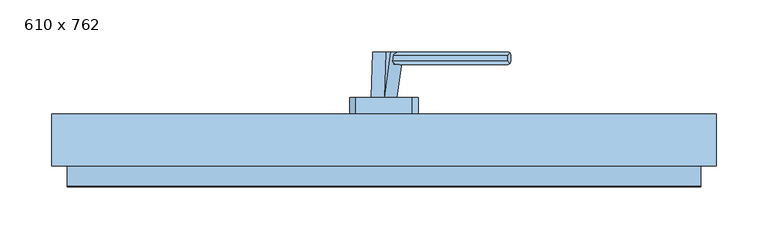
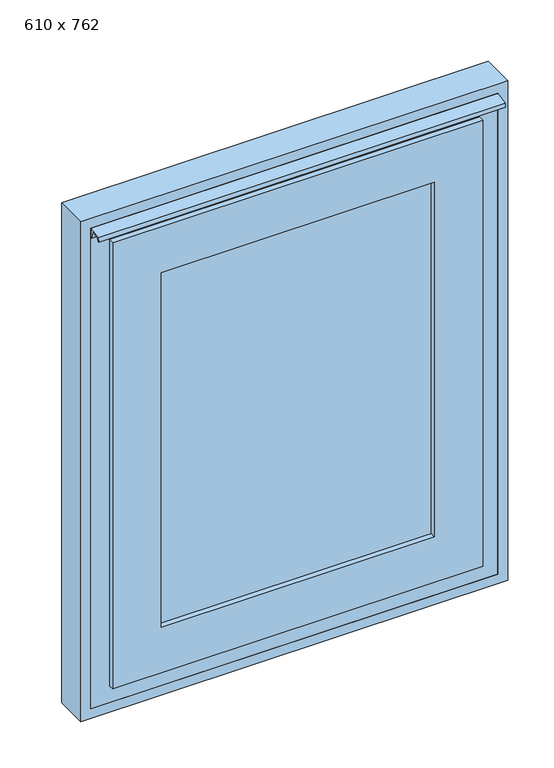
"""IFC4 building model written with IfcOpenShell, lengths in millimetres: window geometry, 610 x 762."""

from ifc_helpers import new_model, si_unit, point, frame, frame_2d, origin, place, context, project, spatial, polyline, circle_curve, ellipse_curve, trimmed, segment, composite_curve, outline, extrude, faceted_brep, source, transform, mapped, element, save
from ifc_brep_helpers import plane_surface, cylinder_surface, extruded_surface, advanced_brep


def window_610_x_762_5077743b(model_context):
    return source(origin(), model_context, "Body", "SolidModel", [
        advanced_brep(
        [(6.2046905, 15.7, 888.0038591), (6.2046905, 15.7, 863.0038591), (1.7209614, 15.7, 863.0038591), (1.7209614, 15.7, 888.0038591), (0.0, -28.3, 888.0038591), (0.0, -28.3, 863.0038591)],
        [
            (0, 1, circle_curve(frame((6.2046905, 15.7, 875.5038591), z_axis=(0.0, 1.0, 0.0), x_axis=(1.0, 0.0, 0.0)), 12.5)),
            (1, 2),
            (2, 3, circle_curve(frame((1.7209614, 15.7, 875.5038591), z_axis=(0.0, 1.0, 0.0), x_axis=(1.0, 0.0, 0.0)), 12.5)),
            (3, 0),
            (4, 5, circle_curve(frame((0.0, -28.3, 875.5038591), z_axis=(0.0, -1.0, 0.0), x_axis=(1.0, 0.0, 0.0)), 12.5)),
            (5, 4, circle_curve(frame((0.0, -28.3, 875.5038591), z_axis=(0.0, -1.0, 0.0), x_axis=(1.0, 0.0, 0.0)), 12.5)),
            (4, 3),
            (2, 5),
            (4, 0),
            (1, 5),
        ],
        [
            plane_surface(frame((3.9628259, 15.7, 875.5038591), z_axis=(0.0, 1.0, 0.0), x_axis=(-1.0, 0.0, 0.0))),
            plane_surface(frame((0.0, -28.3, 875.5038591), z_axis=(0.0, -1.0, 0.0), x_axis=(-1.0, 0.0, 0.0))),
            extruded_surface(trimmed(circle_curve(frame((1.7209614, 15.7, 875.5038591), z_axis=(0.0, -1.0, 0.0), x_axis=(1.0, 0.0, 0.0)), 12.5), [point((1.7209614, 15.7, 888.0038591))], [point((1.7209614, 15.7, 863.0038591))], True, "CARTESIAN"), (-1.7209614, -44.0, 0.0), 44.03364291244014),
            plane_surface(frame((0.0, -28.3, 888.0038591), z_axis=(0.0, 0.0, 1.0), x_axis=(-1.0, 0.0, 0.0))),
            plane_surface(frame((0.0, -28.3, 863.0038591), z_axis=(0.0, 0.0, -1.0), x_axis=(1.0, 0.0, 0.0))),
            extruded_surface(trimmed(circle_curve(frame((6.2046905, 15.7, 875.5038591), z_axis=(0.0, -1.0, 0.0), x_axis=(1.0, 0.0, 0.0)), 12.5), [point((6.2046905, 15.7, 863.0038591))], [point((6.2046905, 15.7, 888.0038591))], True, "CARTESIAN"), (-6.2046905, -44.0, 0.0), 44.43532585905937),
        ],
        [
            (0, [[1, 2, 3, 4]]),
            (1, [[5, 6]]),
            (2, [[7, -3, 8, -5]]),
            (3, [[-7, 9, -4]]),
            (4, [[10, -8, -2]]),
            (5, [[-10, -1, -9, -6]]),
        ],
    ),
        advanced_brep(
        [(122.0, 12.7, 866.0038591), (122.0, 12.7, 885.0038591), (122.0, 6.7, 885.0038591), (122.0, 6.7, 866.0038591), (4.7741708, 15.7, 866.0038591), (113.6581962, 15.7, 866.0038591), (119.0, 15.7, 866.0038591), (121.1213203, 14.8213203, 863.8825388), (119.0, 12.7, 863.0038591), (110.9250215, 12.7, 863.0038591), (4.7741708, 12.7, 863.0038591), (4.7741708, 6.7, 863.0038591), (110.9250215, 6.7, 863.0038591), (119.0, 6.7, 863.0038591), (121.1213203, 4.5786797, 863.8825388), (119.0, 3.7, 866.0038591), (113.6581962, 3.7, 866.0038591), (4.7741708, 3.7, 866.0038591), (119.0, 3.7, 885.0038591), (113.6581962, 3.7, 885.0038591), (4.7741708, 3.7, 885.0038591), (121.1213203, 4.5786797, 887.1251795), (119.0, 6.7, 888.0038591), (110.9250215, 6.7, 888.0038591), (4.7741708, 6.7, 888.0038591), (4.7741708, 12.7, 888.0038591), (110.9250215, 12.7, 888.0038591), (119.0, 12.7, 888.0038591), (121.1213203, 14.8213203, 887.1251795), (119.0, 15.7, 885.0038591), (113.6581962, 15.7, 885.0038591), (4.7741708, 15.7, 885.0038591)],
        [
            (0, 1),
            (1, 2),
            (2, 3),
            (3, 0),
            (4, 5),
            (5, 6),
            (6, 7, ellipse_curve(frame((119.0, 12.7, 866.0038591), z_axis=(-0.70710678118655, 0.0, -0.7071067811865449), x_axis=(0.7071067811865451, 0.0, -0.7071067811865498)), 4.2426407, 3.0)),
            (7, 8, ellipse_curve(frame((119.0, 12.7, 866.0038591), z_axis=(-0.7071067811865427, 0.7071067811865525, 0.0), x_axis=(0.7071067811865522, 0.7071067811865428, 0.0)), 4.2426407, 3.0)),
            (8, 9),
            (9, 10),
            (10, 4, circle_curve(frame((4.7741708, 12.7, 866.0038591), z_axis=(1.0, 0.0, 0.0), x_axis=(0.0, 0.0, 1.0)), 3.0)),
            (11, 12),
            (12, 13),
            (13, 14, ellipse_curve(frame((119.0, 6.7, 866.0038591), z_axis=(-0.7071067811865523, -0.7071067811865426, 0.0), x_axis=(0.7071067811865428, -0.7071067811865522, 0.0)), 4.2426407, 3.0)),
            (14, 15, ellipse_curve(frame((119.0, 6.7, 866.0038591), z_axis=(-0.70710678118655, 0.0, -0.7071067811865449), x_axis=(0.7071067811865451, 0.0, -0.7071067811865498)), 4.2426407, 3.0)),
            (15, 16),
            (16, 17),
            (17, 11, circle_curve(frame((4.7741708, 6.7, 866.0038591), z_axis=(1.0, 0.0, 0.0), x_axis=(0.0, 0.0, 1.0)), 3.0)),
            (15, 18),
            (18, 19),
            (19, 20),
            (20, 17),
            (18, 21, ellipse_curve(frame((119.0, 6.7, 885.0038591), z_axis=(-0.7071067811865449, 0.0, 0.70710678118655), x_axis=(0.7071067811865501, 0.0, 0.7071067811865448)), 4.2426407, 3.0)),
            (21, 22, ellipse_curve(frame((119.0, 6.7, 885.0038591), z_axis=(-0.7071067811865523, -0.7071067811865426, 0.0), x_axis=(0.7071067811865428, -0.7071067811865522, 0.0)), 4.2426407, 3.0)),
            (22, 23),
            (23, 24),
            (24, 20, circle_curve(frame((4.7741708, 6.7, 885.0038591), z_axis=(1.0, 0.0, 0.0), x_axis=(0.0, 0.0, 1.0)), 3.0)),
            (25, 26),
            (26, 27),
            (27, 28, ellipse_curve(frame((119.0, 12.7, 885.0038591), z_axis=(-0.7071067811865427, 0.7071067811865525, 0.0), x_axis=(0.7071067811865522, 0.7071067811865428, 0.0)), 4.2426407, 3.0)),
            (28, 29, ellipse_curve(frame((119.0, 12.7, 885.0038591), z_axis=(-0.7071067811865449, 0.0, 0.70710678118655), x_axis=(0.7071067811865501, 0.0, 0.7071067811865448)), 4.2426407, 3.0)),
            (29, 30),
            (30, 31),
            (31, 25, circle_curve(frame((4.7741708, 12.7, 885.0038591), z_axis=(1.0, 0.0, 0.0), x_axis=(0.0, 0.0, 1.0)), 3.0)),
            (21, 2, ellipse_curve(frame((119.0, 6.7, 885.0038591), z_axis=(0.0, 0.7071067811865451, 0.7071067811865499), x_axis=(0.0, -0.70710678118655, 0.7071067811865451)), 4.2426407, 3.0)),
            (1, 28, ellipse_curve(frame((119.0, 12.7, 885.0038591), z_axis=(0.0, -0.7071067811865499, 0.707106781186545), x_axis=(0.0, -0.7071067811865451, -0.7071067811865498)), 4.2426407, 3.0)),
            (27, 22),
            (7, 0, ellipse_curve(frame((119.0, 12.7, 866.0038591), z_axis=(0.0, -0.7071067811865451, -0.7071067811865499), x_axis=(0.0, -0.70710678118655, 0.7071067811865451)), 4.2426407, 3.0)),
            (3, 14, ellipse_curve(frame((119.0, 6.7, 866.0038591), z_axis=(0.0, 0.7071067811865499, -0.707106781186545), x_axis=(0.0, -0.7071067811865451, -0.7071067811865498)), 4.2426407, 3.0)),
            (13, 8),
            (6, 29),
            (31, 4),
            (10, 11),
            (24, 25),
        ],
        [
            plane_surface(frame((122.0, 15.7, 863.0038591), z_axis=(1.0, 0.0, 0.0), x_axis=(0.0, 0.0, -1.0))),
            cylinder_surface(frame((4.7741708, 12.7, 866.0038591), z_axis=(1.0, 0.0, 0.0), x_axis=(0.0, 0.0, 1.0)), 3.0),
            cylinder_surface(frame((4.7741708, 6.7, 866.0038591), z_axis=(1.0, 0.0, 0.0), x_axis=(0.0, 0.0, 1.0)), 3.0),
            plane_surface(frame((122.0, 3.7, 866.0038591), z_axis=(0.0, -1.0, 0.0), x_axis=(-1.0, 0.0, 0.0))),
            cylinder_surface(frame((4.7741708, 6.7, 885.0038591), z_axis=(1.0, 0.0, 0.0), x_axis=(0.0, 0.0, 1.0)), 3.0),
            cylinder_surface(frame((4.7741708, 12.7, 885.0038591), z_axis=(1.0, 0.0, 0.0), x_axis=(0.0, 0.0, 1.0)), 3.0),
            cylinder_surface(frame((119.0, 3.7, 885.0038591), z_axis=(0.0, -1.0, 0.0), x_axis=(0.0, 0.0, 1.0)), 3.0),
            cylinder_surface(frame((119.0, 3.7, 866.0038591), z_axis=(0.0, -1.0, 0.0), x_axis=(0.0, 0.0, 1.0)), 3.0),
            cylinder_surface(frame((119.0, 6.7, 862.0038591), z_axis=(0.0, 0.0, -1.0), x_axis=(-1.0, 0.0, 0.0)), 3.0),
            cylinder_surface(frame((119.0, 12.7, 862.0038591), z_axis=(0.0, 0.0, -1.0), x_axis=(-1.0, 0.0, 0.0)), 3.0),
            plane_surface(frame((4.7741708, 15.7, 863.0038591), z_axis=(-1.0, 0.0, 0.0), x_axis=(0.0, 0.0, 1.0))),
            plane_surface(frame((122.0, 15.7, 885.0038591), z_axis=(0.0, 1.0, 0.0), x_axis=(-1.0, 0.0, 0.0))),
            plane_surface(frame((122.0, 12.7, 863.0038591), z_axis=(0.0, 0.0, -1.0), x_axis=(-1.0, 0.0, 0.0))),
            plane_surface(frame((122.0, 6.7, 888.0038591), z_axis=(0.0, 0.0, 1.0), x_axis=(-1.0, 0.0, 0.0))),
        ],
        [
            (0, [[1, 2, 3, 4]]),
            (1, [[5, 6, 7, 8, 9, 10, 11]]),
            (2, [[12, 13, 14, 15, 16, 17, 18]]),
            (3, [[-17, -16, 19, 20, 21, 22]]),
            (4, [[-21, -20, 23, 24, 25, 26, 27]]),
            (5, [[28, 29, 30, 31, 32, 33, 34]]),
            (6, [[-24, 35, -2, 36, -30, 37]]),
            (7, [[-8, 38, -4, 39, -14, 40]]),
            (8, [[-35, -23, -19, -15, -39, -3]]),
            (9, [[-38, -7, 41, -31, -36, -1]]),
            (10, [[42, -11, 43, -18, -22, -27, 44, -34]]),
            (11, [[-33, -32, -41, -6, -5, -42]]),
            (12, [[-10, -9, -40, -13, -12, -43]]),
            (13, [[-26, -25, -37, -29, -28, -44]]),
        ],
    ),
        extrude(outline(composite_curve([segment(polyline([(883.0038591, -33.0), (868.0038591, -33.0)]), True, "CONTINUOUS"), segment(trimmed(circle_curve(frame_2d((868.0038591, -27.0)), 6.0), [point((868.0038591, -33.0))], [point((862.0038591, -27.0))], False, "CARTESIAN"), True, "CONTINUOUS"), segment(polyline([(862.0038591, -27.0), (862.0038591, 27.0)]), True, "CONTINUOUS"), segment(trimmed(circle_curve(frame_2d((868.0038591, 27.0)), 6.0), [point((862.0038591, 27.0))], [point((868.0038591, 33.0))], False, "CARTESIAN"), True, "CONTINUOUS"), segment(polyline([(868.0038591, 33.0), (883.0038591, 33.0)]), True, "CONTINUOUS"), segment(trimmed(circle_curve(frame_2d((883.0038591, 27.0)), 6.0), [point((883.0038591, 33.0))], [point((889.0038591, 27.0))], False, "CARTESIAN"), True, "CONTINUOUS"), segment(polyline([(889.0038591, 27.0), (889.0038591, -27.0)]), True, "CONTINUOUS"), segment(trimmed(circle_curve(frame_2d((883.0038591, -27.0)), 6.0), [point((889.0038591, -27.0))], [point((883.0038591, -33.0))], False, "CARTESIAN"), True, "CONTINUOUS")], self_intersect=False)), frame((0.0, -44.3, 0.0), z_axis=(0.0, 1.0, 0.0), x_axis=(0.0, 0.0, 1.0)), (0.0, 0.0, 1.0), 16.0),
        extrude(outline(polyline([(1577.0, -319.8), (785.0, -319.8), (785.0, 319.8), (1577.0, 319.8), (1577.0, -319.8)]), holes=[polyline([(800.0, -304.8), (1562.0, -304.8), (1562.0, 304.8), (800.0, 304.8), (800.0, -304.8)])]), frame((0.0, -94.3, 0.0), z_axis=(0.0, 1.0, 0.0), x_axis=(0.0, 0.0, 1.0)), (0.0, 0.0, 1.0), 50.0),
        faceted_brep([(-304.8, -44.3, 1562.0), (-304.8, -44.3, 800.0), (-304.8, -94.3, 800.0), (-304.8, -94.3, 1562.0), (-271.3, -94.3, 1528.5), (-271.3, -94.3, 833.5), (-271.3, -49.5, 833.5), (-271.3, -49.5, 1528.5), (-249.3, -49.5, 1506.5), (-249.3, -49.5, 855.5), (-249.3, -44.3, 855.5), (-249.3, -44.3, 1506.5), (304.8, -44.3, 800.0), (304.8, -94.3, 800.0), (271.3, -94.3, 833.5), (271.3, -49.5, 833.5), (249.3, -49.5, 855.5), (249.3, -44.3, 855.5), (304.8, -44.3, 1562.0), (304.8, -94.3, 1562.0), (271.3, -94.3, 1528.5), (271.3, -49.5, 1528.5), (249.3, -49.5, 1506.5), (249.3, -44.3, 1506.5)], [[[0, 1, 2, 3]], [[4, 5, 6, 7]], [[8, 9, 10, 11]], [[1, 12, 13, 2]], [[5, 14, 15, 6]], [[9, 16, 17, 10]], [[12, 18, 19, 13]], [[14, 20, 21, 15]], [[16, 22, 23, 17]], [[18, 0, 3, 19]], [[3, 2, 13, 19], [5, 4, 20, 14]], [[20, 4, 7, 21]], [[7, 6, 15, 21], [9, 8, 22, 16]], [[22, 8, 11, 23]], [[1, 0, 18, 12], [11, 10, 17, 23]]]),
        extrude(outline(polyline([(-220.8, -70.8), (220.8, -70.8), (220.8, -94.8), (-220.8, -94.8), (-220.8, -70.8)])), frame((0.0, 0.0, 884.0), z_axis=(0.0, 0.0, 1.0), x_axis=(1.0, 0.0, 0.0)), (0.0, 0.0, 1.0), 594.0),
        faceted_brep([(277.3, -103.3, 1534.5), (277.3, -103.3, 827.5), (277.3, -94.3, 827.5), (277.3, -94.3, 1534.5), (204.8, -94.8, 1462.0), (204.8, -94.8, 900.0), (204.8, -103.3, 900.0), (204.8, -103.3, 1462.0), (220.8, -70.8, 1478.0), (220.8, -70.8, 884.0), (220.8, -94.8, 884.0), (220.8, -94.8, 1478.0), (208.8, -44.3, 1466.0), (208.8, -44.3, 896.0), (208.8, -70.8, 896.0), (208.8, -70.8, 1466.0), (244.3, -49.5, 1501.5), (244.3, -49.5, 860.5), (244.3, -44.3, 860.5), (244.3, -44.3, 1501.5), (259.9392195, -94.3, 1517.1392195), (259.9392195, -94.3, 844.8607805), (259.9392195, -49.5, 844.8607805), (259.9392195, -49.5, 1517.1392195), (-277.3, -103.3, 827.5), (-277.3, -94.3, 827.5), (-204.8, -94.8, 900.0), (-204.8, -103.3, 900.0), (-220.8, -70.8, 884.0), (-220.8, -94.8, 884.0), (-208.8, -44.3, 896.0), (-208.8, -70.8, 896.0), (-244.3, -49.5, 860.5), (-244.3, -44.3, 860.5), (-259.9392195, -94.3, 844.8607805), (-259.9392195, -49.5, 844.8607805), (-277.3, -103.3, 1534.5), (-277.3, -94.3, 1534.5), (-204.8, -94.8, 1462.0), (-204.8, -103.3, 1462.0), (-220.8, -70.8, 1478.0), (-220.8, -94.8, 1478.0), (-208.8, -44.3, 1466.0), (-208.8, -70.8, 1466.0), (-244.3, -49.5, 1501.5), (-244.3, -44.3, 1501.5), (-259.9392195, -94.3, 1517.1392195), (-259.9392195, -49.5, 1517.1392195)], [[[0, 1, 2, 3]], [[4, 5, 6, 7]], [[8, 9, 10, 11]], [[12, 13, 14, 15]], [[16, 17, 18, 19]], [[20, 21, 22, 23]], [[1, 24, 25, 2]], [[5, 26, 27, 6]], [[9, 28, 29, 10]], [[13, 30, 31, 14]], [[17, 32, 33, 18]], [[21, 34, 35, 22]], [[24, 36, 37, 25]], [[26, 38, 39, 27]], [[28, 40, 41, 29]], [[30, 42, 43, 31]], [[32, 44, 45, 33]], [[34, 46, 47, 35]], [[36, 0, 3, 37]], [[1, 0, 36, 24], [7, 6, 27, 39]], [[38, 4, 7, 39]], [[11, 10, 29, 41], [5, 4, 38, 26]], [[40, 8, 11, 41]], [[9, 8, 40, 28], [15, 14, 31, 43]], [[42, 12, 15, 43]], [[19, 18, 33, 45], [13, 12, 42, 30]], [[44, 16, 19, 45]], [[23, 22, 35, 47], [17, 16, 44, 32]], [[46, 20, 23, 47]], [[3, 2, 25, 37], [21, 20, 46, 34]]]),
        extrude(outline(polyline([(-94.3, 1547.0), (-95.9649679, 1547.0), (-98.5146457, 1559.11097), (-111.751709, 1556.3242199), (-113.0, 1552.0), (-114.5, 1552.0), (-113.5, 1558.0), (-94.3, 1562.0421053), (-94.3, 1547.0)])), frame((-304.8, 0.0, 0.0), z_axis=(1.0, 0.0, 0.0), x_axis=(0.0, 1.0, 0.0)), (0.0, 0.0, 1.0), 609.6),
    ])


if __name__ == "__main__":
    model = new_model("IFC4")
    model_context = context("Model", 3, world=origin())
    ifc_project = project(units=[si_unit("LENGTHUNIT", "METRE", prefix="MILLI")], contexts=[model_context])
    site = spatial("IfcSite", under=ifc_project)
    building = spatial("IfcBuilding", under=site)
    placement = place(None, origin())
    window_610_x_762_shape = window_610_x_762_5077743b(model_context)
    element("IfcWindow", 1, ObjectType="610 x 762", at=placement, inside=building, context=model_context, shape_type="MappedRepresentation", body=[
        mapped(window_610_x_762_shape, transform((0.0, 0.0, 0.0), x_axis=(1.0, 0.0, 0.0), y_axis=(0.0, 1.0, 0.0), z_axis=(0.0, 0.0, 1.0))),
    ])
    save(model, "model.ifc")

# Revit data of these elements
# Type "610 x 762"
#   Type Mark = "18"
#   Water resistance = "up to Class E1050, PN-EN 12208:2001"
#   URL = "https://aluprof.com/en/architects/offer/window-and-door-systems/mb-59s-casement-mb-59s-casement-hi"
#   Type IFC Predefined Type = "NOTDEFINED"
#   Resistance to wind load = "up to Class C5, PN-EN 12210:2016"
#   Operation = "SingleTopHungCasement"
#   Opening type = "Top-hung casement opening outwards"
#   Model = "MB-59S Casement"
#   ManufacturerSustainabilityPolicyURL = "https://aluprof.eu/en/company/sustainable-development"
#   Manufacturer = "ALUPROF SA"
#   Keynote = "08511300"
#   IfcExportType = "NOTDEFINED"
#   IfcExportAs = "IfcWindowType"
#   Hardware [instance default] = ""
#   Handle type [instance default] = ""
#   Glazing construction = "4/16/4"
#   Export Type to IFC As = "IfcWindowType"
#   Description = "Single top-hung casement opening outwards"
#   Content of the recyclate in the material = "69.2%"
#   COBie.Type.Name = "MB-59S Casement"
#   COBie.Type.Manufacturer = "ALUPROF SA\r\nALUPROF S.A.\r\nALUPROF S.A."
#   Assembly Code = "B2020110"
#   Analytic Construction = "<None>"
#   Air permeability = "up to Class 4, PN-EN 12207:2001"
#   Thermal insulation = 0.299387 BTU/(h·ft²·°F)
#   Sash thickness = 0' - 2.32283"
#   Rough Width = 2' - 1.1811"
#   Rough Height = 2' - 7.1811"
#   Reference line height [instance default] = 0' - 0"
#   Opening angle [instance default] = 0.00°
#   Mounting space = 0' - 0.59055"
#   Height = 2' - 6"
#   Glazing area = 2.82349 SF
#   Frame thickness = 0' - 1.9685"
#   Exterior wall face offset = 0' - 0.7874"
#   Sill Height = 2' - 7.49606"
#   Width = 2' - 0"
#   Warm installation [instance default] = yes
#   Thermal variant HI = no
#   Schedule No. [instance default] = 1
#   IsWindowOpen [instance default] = no
#   IsExternal = yes
#   Define Thermal Properties by = 1
#   COBie.Type = yes
#   COBie = yes
#   Wall Closure = (empty or 0)
